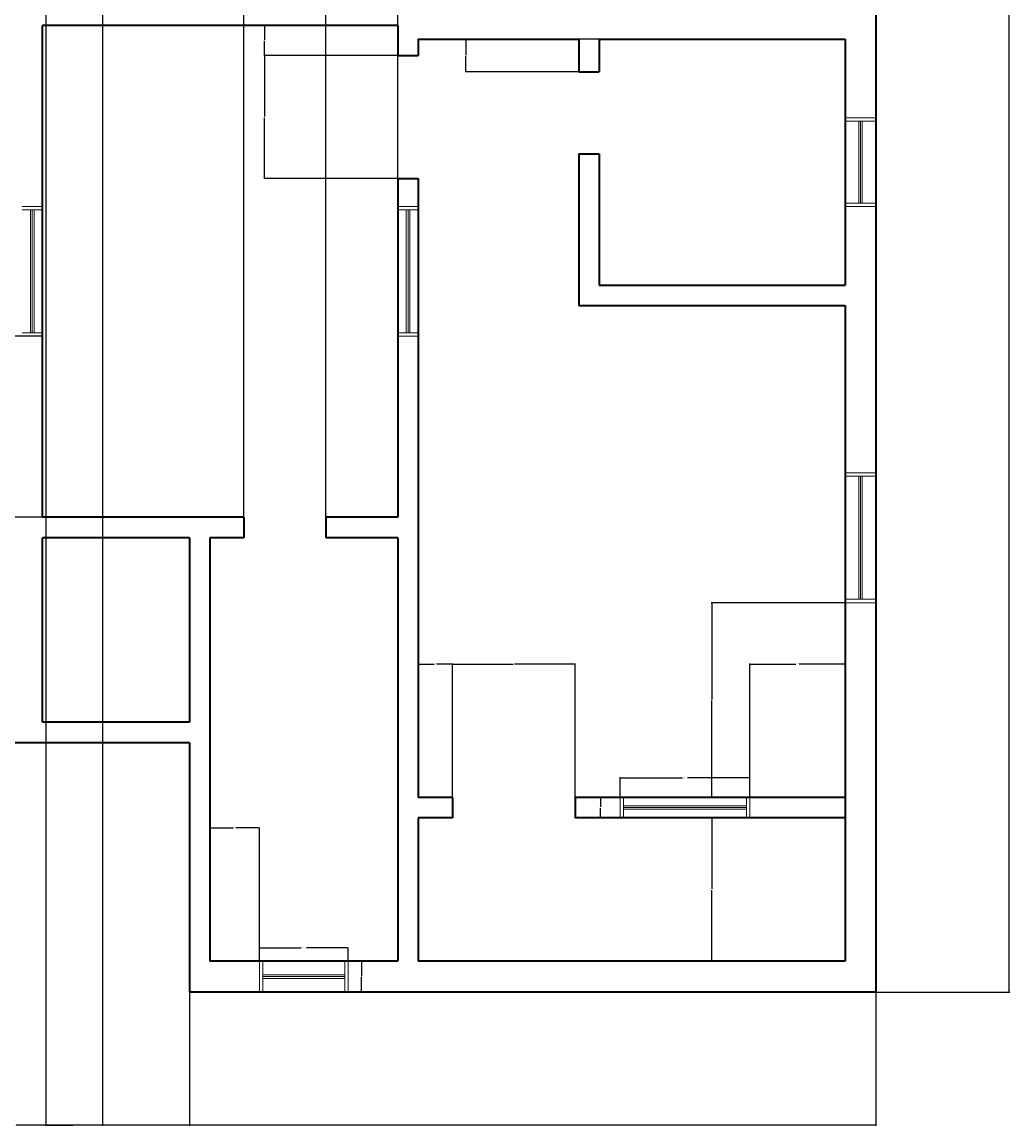
# Model space of a CAD drawing. Units: inches. Extents: x -7288 to -6705, y 7169 to 8028.
# Tile 2 of 5: x -6995 to -6706, y 7169 to 7493. Entities that reach past the tile are written whole.
import ezdxf

# ---------------------------------------------------------------- set-up
doc = ezdxf.new("R2010")
doc.units = ezdxf.units.IN
for name, color, linetype, lineweight in [('A-ANNO-DIMS', 2, 'Continuous', 18), ('A-GLAZ', 2, 'Continuous', 18), ('A-WALL', 1, 'Continuous', 35)]:
    doc.layers.add(name, color=color, linetype=linetype, lineweight=lineweight)
doc.styles.get("Standard").update_dxf_attribs({"font": 'arial.ttf'})
doc.dimstyles.get("Standard").update_dxf_attribs({"dimtxt": 0.18, "dimasz": 0.18, "dimexe": 0.18, "dimexo": 0.0625, "dimgap": 0.09, "dimtad": 0, "dimtih": 1, "dimtoh": 1, "dimdec": 4, "dimzin": 0, "dimdsep": 46, "dimtxsty": 'Standard', "dimcen": 0.09, "dimadec": 0, "dimazin": 0, "dimtfac": 1, "dimtdec": 4, "dimtofl": 0, "dimtmove": 0, "dimatfit": 3, "dimfxl": 1, "dimtolj": 1, "dimtzin": 0, "dimarcsym": 0})

# ---------------------------------------------------------------- blocks, each defined once
blk = doc.blocks.new('WIN-36IN-WALL9')
for p, q in [((0, 38), (9, 38)), ((0, 37), (9, 37)), ((4, 1), (4, 37)), ((4.5, 1), (4.5, 37)), ((5, 1), (5, 37)), ((0, 1), (9, 1)), ((0, 0), (9, 0))]:
    blk.add_line(p, q)
blk = doc.blocks.new('WIN-24IN-WALL9')
for p, q in [((0, 26), (9, 26)), ((0, 25), (9, 25)), ((4, 1), (4, 25)), ((4.5, 1), (4.5, 25)), ((5, 1), (5, 25)), ((0, 1), (9, 1)), ((0, 0), (9, 0))]:
    blk.add_line(p, q)
blk = doc.blocks.new('WIN-36IN-WALL6')
for p, q in [((0, 6), (0, 0)), ((1, 6), (1, 0)), ((1, 3.5), (37, 3.5)), ((37, 6), (37, 0)), ((38, 6), (38, 0)), ((1, 3), (37, 3)), ((1, 2.5), (37, 2.5))]:
    blk.add_line(p, q)
blk = doc.blocks.new('*D89')
at = {"layer": 'A-ANNO-DIMS', "color": 0, "lineweight": -2, "transparency": 16777216}
for p, q in [((-6925.34, 7217.59), (-6925.34, 7221.61)), ((-6925.16, 7221.43), (-6913.1, 7221.43)), ((-6899.52, 7221.43), (-6911.58, 7221.43)), ((-6899.34, 7217.59), (-6899.34, 7221.61))]:
    blk.add_line(p, q, dxfattribs=at)
at = {"layer": 'A-ANNO-DIMS', "color": 0, "transparency": 16777216}
for points in [[(-6925.16, 7221.46), (-6925.16, 7221.4), (-6925.34, 7221.43)], [(-6899.52, 7221.46), (-6899.52, 7221.4), (-6899.34, 7221.43)]]:
    blk.add_solid(points, dxfattribs=at)
at = {"layer": 'Defpoints', "color": 0, "transparency": 16777216}
for p in [(-6899.34, 7221.43), (-6925.34, 7217.53), (-6899.34, 7217.53)]:
    blk.add_point(p, dxfattribs=at)
at = {"layer": 'A-ANNO-DIMS', "color": 0, "transparency": 16777216, "insert": (-6912.34, 7221.43), "char_height": 0.18, "attachment_point": 5}
blk.add_mtext('\\A1;W2 26 TYP.', dxfattribs=at)
blk = doc.blocks.new('*D90')
at = {"layer": 'A-ANNO-DIMS', "color": 0, "lineweight": -2, "transparency": 16777216}
for p, q in [((-6899.28, 7217.53), (-6895.26, 7217.53)), ((-6895.44, 7217.35), (-6895.44, 7213.21)), ((-6895.44, 7208.71), (-6895.44, 7212.85)), ((-6899.28, 7208.53), (-6895.26, 7208.53))]:
    blk.add_line(p, q, dxfattribs=at)
at = {"layer": 'A-ANNO-DIMS', "color": 0, "transparency": 16777216}
for points in [[(-6895.47, 7217.35), (-6895.41, 7217.35), (-6895.44, 7217.53)], [(-6895.47, 7208.71), (-6895.41, 7208.71), (-6895.44, 7208.53)]]:
    blk.add_solid(points, dxfattribs=at)
at = {"layer": 'Defpoints', "color": 0, "transparency": 16777216}
for p in [(-6899.34, 7217.53), (-6899.34, 7208.53), (-6895.44, 7208.53)]:
    blk.add_point(p, dxfattribs=at)
at = {"layer": 'A-ANNO-DIMS', "color": 0, "transparency": 16777216, "insert": (-6895.44, 7213.03), "char_height": 0.18, "attachment_point": 5}
blk.add_mtext('\\A1;9 TYP.', dxfattribs=at)
blk = doc.blocks.new('*D91')
at = {"layer": 'A-ANNO-DIMS', "color": 0, "lineweight": -2, "transparency": 16777216}
for p, q in [((-6819.77, 7265.59), (-6819.77, 7271.41)), ((-6819.59, 7271.23), (-6801.52, 7271.23)), ((-6781.95, 7271.23), (-6800.01, 7271.23)), ((-6781.77, 7265.59), (-6781.77, 7271.41))]:
    blk.add_line(p, q, dxfattribs=at)
at = {"layer": 'A-ANNO-DIMS', "color": 0, "transparency": 16777216}
for points in [[(-6819.59, 7271.26), (-6819.59, 7271.2), (-6819.77, 7271.23)], [(-6781.95, 7271.26), (-6781.95, 7271.2), (-6781.77, 7271.23)]]:
    blk.add_solid(points, dxfattribs=at)
at = {"layer": 'Defpoints', "color": 0, "transparency": 16777216}
for p in [(-6781.77, 7271.23), (-6819.77, 7265.53), (-6781.77, 7265.53)]:
    blk.add_point(p, dxfattribs=at)
at = {"layer": 'A-ANNO-DIMS', "color": 0, "transparency": 16777216, "insert": (-6800.77, 7271.23), "char_height": 0.18, "attachment_point": 5}
blk.add_mtext('\\A1;W3 38 TYP.', dxfattribs=at)
blk = doc.blocks.new('*D92')
at = {"layer": 'A-ANNO-DIMS', "color": 0, "lineweight": -2, "transparency": 16777216}
for p, q in [((-6819.83, 7265.53), (-6825.65, 7265.53)), ((-6825.47, 7265.35), (-6825.47, 7262.71)), ((-6819.83, 7259.53), (-6825.65, 7259.53)), ((-6825.47, 7259.71), (-6825.47, 7262.35))]:
    blk.add_line(p, q, dxfattribs=at)
at = {"layer": 'A-ANNO-DIMS', "color": 0, "transparency": 16777216}
for points in [[(-6825.5, 7265.35), (-6825.44, 7265.35), (-6825.47, 7265.53)], [(-6825.5, 7259.71), (-6825.44, 7259.71), (-6825.47, 7259.53)]]:
    blk.add_solid(points, dxfattribs=at)
at = {"layer": 'Defpoints', "color": 0, "transparency": 16777216}
for p in [(-6825.47, 7265.53), (-6819.77, 7265.53), (-6819.77, 7259.53)]:
    blk.add_point(p, dxfattribs=at)
at = {"layer": 'A-ANNO-DIMS', "color": 0, "transparency": 16777216, "insert": (-6825.47, 7262.53), "char_height": 0.18, "attachment_point": 5}
blk.add_mtext('\\A1;6 TYP.', dxfattribs=at)
blk = doc.blocks.new('*D93')
at = {"layer": 'A-ANNO-DIMS', "color": 0, "lineweight": -2, "transparency": 16777216}
for p, q in [((-7248.84, 7208.47), (-7248.84, 7169.32)), ((-6744.84, 7208.47), (-6744.84, 7169.32)), ((-7248.66, 7169.5), (-6997.13, 7169.5)), ((-6745.02, 7169.5), (-6996.55, 7169.5))]:
    blk.add_line(p, q, dxfattribs=at)
at = {"layer": 'A-ANNO-DIMS', "color": 0, "transparency": 16777216}
for points in [[(-7248.66, 7169.53), (-7248.66, 7169.47), (-7248.84, 7169.5)], [(-6745.02, 7169.53), (-6745.02, 7169.47), (-6744.84, 7169.5)]]:
    blk.add_solid(points, dxfattribs=at)
at = {"layer": 'Defpoints', "color": 0, "transparency": 16777216}
for p in [(-7248.84, 7208.53), (-6744.84, 7208.53), (-6744.84, 7169.5)]:
    blk.add_point(p, dxfattribs=at)
at = {"layer": 'A-ANNO-DIMS', "color": 0, "transparency": 16777216, "insert": (-6996.84, 7169.5), "char_height": 0.18, "attachment_point": 5}
blk.add_mtext('\\A1;504', dxfattribs=at)
blk = doc.blocks.new('*D94')
at = {"layer": 'A-ANNO-DIMS', "color": 0, "lineweight": -2, "transparency": 16777216}
for p, q in [((-6802.78, 7988.53), (-6705.63, 7988.53)), ((-6705.81, 7988.35), (-6705.81, 7598.71)), ((-6705.81, 7208.71), (-6705.81, 7598.35)), ((-6744.78, 7208.53), (-6705.63, 7208.53))]:
    blk.add_line(p, q, dxfattribs=at)
at = {"layer": 'A-ANNO-DIMS', "color": 0, "transparency": 16777216}
for points in [[(-6705.84, 7988.35), (-6705.78, 7988.35), (-6705.81, 7988.53)], [(-6705.84, 7208.71), (-6705.78, 7208.71), (-6705.81, 7208.53)]]:
    blk.add_solid(points, dxfattribs=at)
at = {"layer": 'Defpoints', "color": 0, "transparency": 16777216}
for p in [(-6802.84, 7988.53), (-6705.81, 7988.53), (-6744.84, 7208.53)]:
    blk.add_point(p, dxfattribs=at)
at = {"layer": 'A-ANNO-DIMS', "color": 0, "transparency": 16777216, "insert": (-6705.81, 7598.53), "char_height": 0.18, "attachment_point": 5}
blk.add_mtext('\\A1;780', dxfattribs=at)
blk = doc.blocks.new('*D101')
at = {"layer": 'A-ANNO-DIMS', "color": 0, "lineweight": -2, "transparency": 16777216}
for p, q in [((-7047.84, 7208.47), (-7047.84, 7169.32)), ((-6945.84, 7208.47), (-6945.84, 7169.32)), ((-7047.66, 7169.5), (-6997.12, 7169.5)), ((-6946.02, 7169.5), (-6996.56, 7169.5))]:
    blk.add_line(p, q, dxfattribs=at)
at = {"layer": 'A-ANNO-DIMS', "color": 0, "transparency": 16777216}
for points in [[(-7047.66, 7169.53), (-7047.66, 7169.47), (-7047.84, 7169.5)], [(-6946.02, 7169.53), (-6946.02, 7169.47), (-6945.84, 7169.5)]]:
    blk.add_solid(points, dxfattribs=at)
at = {"layer": 'Defpoints', "color": 0, "transparency": 16777216}
for p in [(-7047.84, 7208.53), (-6945.84, 7208.53), (-6945.84, 7169.5)]:
    blk.add_point(p, dxfattribs=at)
at = {"layer": 'A-ANNO-DIMS', "color": 0, "transparency": 16777216, "insert": (-6996.84, 7169.5), "char_height": 0.18, "attachment_point": 5}
blk.add_mtext('\\A1;102', dxfattribs=at)
blk = doc.blocks.new('*D115')
at = {"layer": 'A-ANNO-DIMS', "color": 0, "lineweight": -2, "transparency": 16777216}
for p, q in [((-6971.26, 7899.49), (-6971.26, 7169.32)), ((-6987.84, 7886.47), (-6987.84, 7169.32)), ((-6987.66, 7169.5), (-6980.01, 7169.5)), ((-6971.44, 7169.5), (-6979.1, 7169.5))]:
    blk.add_line(p, q, dxfattribs=at)
at = {"layer": 'A-ANNO-DIMS', "color": 0, "transparency": 16777216}
for points in [[(-6987.66, 7169.53), (-6987.66, 7169.47), (-6987.84, 7169.5)], [(-6971.44, 7169.53), (-6971.44, 7169.47), (-6971.26, 7169.5)]]:
    blk.add_solid(points, dxfattribs=at)
at = {"layer": 'Defpoints', "color": 0, "transparency": 16777216}
for p in [(-6971.26, 7899.55), (-6987.84, 7886.53), (-6971.26, 7169.5)]:
    blk.add_point(p, dxfattribs=at)
at = {"layer": 'A-ANNO-DIMS', "color": 0, "transparency": 16777216, "insert": (-6979.55, 7169.5), "char_height": 0.18, "attachment_point": 5}
blk.add_mtext('\\A1;16.578', dxfattribs=at)
blk = doc.blocks.new('*D143')
at = {"layer": 'A-ANNO-DIMS', "color": 0, "lineweight": -2, "transparency": 16777216}
for p, q in [((-6753.9, 7259.53), (-6793.05, 7259.53)), ((-6792.87, 7259.35), (-6792.87, 7238.71)), ((-6792.87, 7217.71), (-6792.87, 7238.35)), ((-6753.9, 7217.53), (-6793.05, 7217.53))]:
    blk.add_line(p, q, dxfattribs=at)
at = {"layer": 'A-ANNO-DIMS', "color": 0, "transparency": 16777216}
for points in [[(-6792.9, 7259.35), (-6792.84, 7259.35), (-6792.87, 7259.53)], [(-6792.9, 7217.71), (-6792.84, 7217.71), (-6792.87, 7217.53)]]:
    blk.add_solid(points, dxfattribs=at)
at = {"layer": 'Defpoints', "color": 0, "transparency": 16777216}
for p in [(-6792.87, 7259.53), (-6753.84, 7259.53), (-6753.84, 7217.53)]:
    blk.add_point(p, dxfattribs=at)
at = {"layer": 'A-ANNO-DIMS', "color": 0, "transparency": 16777216, "insert": (-6792.87, 7238.53), "char_height": 0.18, "attachment_point": 5}
blk.add_mtext('\\A1;42', dxfattribs=at)
blk = doc.blocks.new('*D153')
at = {"layer": 'A-ANNO-DIMS', "color": 0, "lineweight": -2, "transparency": 16777216}
for p, q in [((-6753.9, 7322.53), (-6793.05, 7322.53)), ((-6792.87, 7322.35), (-6792.87, 7294.21)), ((-6792.87, 7265.71), (-6792.87, 7293.85)), ((-6753.9, 7265.53), (-6793.05, 7265.53))]:
    blk.add_line(p, q, dxfattribs=at)
at = {"layer": 'A-ANNO-DIMS', "color": 0, "transparency": 16777216}
for points in [[(-6792.9, 7322.35), (-6792.84, 7322.35), (-6792.87, 7322.53)], [(-6792.9, 7265.71), (-6792.84, 7265.71), (-6792.87, 7265.53)]]:
    blk.add_solid(points, dxfattribs=at)
at = {"layer": 'Defpoints', "color": 0, "transparency": 16777216}
for p in [(-6792.87, 7322.53), (-6753.84, 7322.53), (-6753.84, 7265.53)]:
    blk.add_point(p, dxfattribs=at)
at = {"layer": 'A-ANNO-DIMS', "color": 0, "transparency": 16777216, "insert": (-6792.87, 7294.03), "char_height": 0.18, "attachment_point": 5}
blk.add_mtext('\\A1;57', dxfattribs=at)
blk = doc.blocks.new('*D154')
at = {"layer": 'A-ANNO-DIMS', "color": 0, "lineweight": -2, "transparency": 16777216}
for p, q in [((-6905.9, 7347.59), (-6905.9, 8027.74)), ((-6905.72, 8027.56), (-6895.77, 8027.56)), ((-6885.02, 8027.56), (-6894.97, 8027.56)), ((-6884.84, 7347.59), (-6884.84, 8027.74))]:
    blk.add_line(p, q, dxfattribs=at)
at = {"layer": 'A-ANNO-DIMS', "color": 0, "transparency": 16777216}
for points in [[(-6905.72, 8027.59), (-6905.72, 8027.53), (-6905.9, 8027.56)], [(-6885.02, 8027.59), (-6885.02, 8027.53), (-6884.84, 8027.56)]]:
    blk.add_solid(points, dxfattribs=at)
at = {"layer": 'Defpoints', "color": 0, "transparency": 16777216}
for p in [(-6884.84, 8027.56), (-6905.9, 7347.53), (-6884.84, 7347.53)]:
    blk.add_point(p, dxfattribs=at)
at = {"layer": 'A-ANNO-DIMS', "color": 0, "transparency": 16777216, "insert": (-6895.37, 8027.56), "char_height": 0.18, "attachment_point": 5}
blk.add_mtext('\\A1;21.06', dxfattribs=at)
blk = doc.blocks.new('*D155')
at = {"layer": 'A-ANNO-DIMS', "color": 0, "lineweight": -2, "transparency": 16777216}
for p, q in [((-6929.9, 7347.59), (-6929.9, 8027.74)), ((-6929.72, 8027.56), (-6918.12, 8027.56)), ((-6906.08, 8027.56), (-6917.68, 8027.56)), ((-6905.9, 7347.59), (-6905.9, 8027.74))]:
    blk.add_line(p, q, dxfattribs=at)
at = {"layer": 'A-ANNO-DIMS', "color": 0, "transparency": 16777216}
for points in [[(-6929.72, 8027.59), (-6929.72, 8027.53), (-6929.9, 8027.56)], [(-6906.08, 8027.59), (-6906.08, 8027.53), (-6905.9, 8027.56)]]:
    blk.add_solid(points, dxfattribs=at)
at = {"layer": 'Defpoints', "color": 0, "transparency": 16777216}
for p in [(-6905.9, 8027.56), (-6929.9, 7347.53), (-6905.9, 7347.53)]:
    blk.add_point(p, dxfattribs=at)
at = {"layer": 'A-ANNO-DIMS', "color": 0, "transparency": 16777216, "insert": (-6917.9, 8027.56), "char_height": 0.18, "attachment_point": 5}
blk.add_mtext('\\A1;24', dxfattribs=at)
blk = doc.blocks.new('*D159')
at = {"layer": 'A-ANNO-DIMS', "color": 0, "lineweight": -2, "transparency": 16777216}
for p, q in [((-6939.84, 7217.59), (-6939.84, 7256.74)), ((-6939.66, 7256.56), (-6932.91, 7256.56)), ((-6925.52, 7256.56), (-6932.27, 7256.56)), ((-6925.34, 7217.59), (-6925.34, 7256.74))]:
    blk.add_line(p, q, dxfattribs=at)
at = {"layer": 'A-ANNO-DIMS', "color": 0, "transparency": 16777216}
for points in [[(-6939.66, 7256.59), (-6939.66, 7256.53), (-6939.84, 7256.56)], [(-6925.52, 7256.59), (-6925.52, 7256.53), (-6925.34, 7256.56)]]:
    blk.add_solid(points, dxfattribs=at)
at = {"layer": 'Defpoints', "color": 0, "transparency": 16777216}
for p in [(-6925.34, 7256.56), (-6939.84, 7217.53), (-6925.34, 7217.53)]:
    blk.add_point(p, dxfattribs=at)
at = {"layer": 'A-ANNO-DIMS', "color": 0, "transparency": 16777216, "insert": (-6932.59, 7256.56), "char_height": 0.18, "attachment_point": 5}
blk.add_mtext('\\A1;14.5', dxfattribs=at)
blk = doc.blocks.new('*D160')
at = {"layer": 'A-ANNO-DIMS', "color": 0, "lineweight": -2, "transparency": 16777216}
for p, q in [((-6988.9, 7400.53), (-7028.05, 7400.53)), ((-7027.87, 7400.35), (-7027.87, 7374.21)), ((-7027.87, 7347.71), (-7027.87, 7373.85)), ((-6988.9, 7347.53), (-7028.05, 7347.53))]:
    blk.add_line(p, q, dxfattribs=at)
at = {"layer": 'A-ANNO-DIMS', "color": 0, "transparency": 16777216}
for points in [[(-7027.9, 7400.35), (-7027.84, 7400.35), (-7027.87, 7400.53)], [(-7027.9, 7347.71), (-7027.84, 7347.71), (-7027.87, 7347.53)]]:
    blk.add_solid(points, dxfattribs=at)
at = {"layer": 'Defpoints', "color": 0, "transparency": 16777216}
for p in [(-7027.87, 7400.53), (-6988.84, 7400.53), (-6988.84, 7347.53)]:
    blk.add_point(p, dxfattribs=at)
at = {"layer": 'A-ANNO-DIMS', "color": 0, "transparency": 16777216, "insert": (-7027.87, 7374.03), "char_height": 0.18, "attachment_point": 5}
blk.add_mtext('\\A1;53', dxfattribs=at)
blk = doc.blocks.new('*D162')
at = {"layer": 'A-ANNO-DIMS', "color": 0, "lineweight": -2, "transparency": 16777216}
for p, q in [((-6781.77, 7265.59), (-6781.77, 7304.74)), ((-6781.59, 7304.56), (-6768.27, 7304.56)), ((-6754.02, 7304.56), (-6767.34, 7304.56)), ((-6753.84, 7265.59), (-6753.84, 7304.74))]:
    blk.add_line(p, q, dxfattribs=at)
at = {"layer": 'A-ANNO-DIMS', "color": 0, "transparency": 16777216}
for points in [[(-6781.59, 7304.59), (-6781.59, 7304.53), (-6781.77, 7304.56)], [(-6754.02, 7304.59), (-6754.02, 7304.53), (-6753.84, 7304.56)]]:
    blk.add_solid(points, dxfattribs=at)
at = {"layer": 'Defpoints', "color": 0, "transparency": 16777216}
for p in [(-6753.84, 7304.56), (-6781.77, 7265.53), (-6753.84, 7265.53)]:
    blk.add_point(p, dxfattribs=at)
at = {"layer": 'A-ANNO-DIMS', "color": 0, "transparency": 16777216, "insert": (-6767.8, 7304.56), "char_height": 0.18, "attachment_point": 5}
blk.add_mtext('\\A1;27.925', dxfattribs=at)
blk = doc.blocks.new('*D167')
at = {"layer": 'A-ANNO-DIMS', "color": 0, "lineweight": -2, "transparency": 16777216}
for p, q in [((-6884.9, 7482.7), (-6924.05, 7482.7)), ((-6923.87, 7482.52), (-6923.87, 7464.88)), ((-6923.87, 7446.88), (-6923.87, 7464.52)), ((-6884.9, 7446.7), (-6924.05, 7446.7))]:
    blk.add_line(p, q, dxfattribs=at)
at = {"layer": 'A-ANNO-DIMS', "color": 0, "transparency": 16777216}
for points in [[(-6923.9, 7482.52), (-6923.84, 7482.52), (-6923.87, 7482.7)], [(-6923.9, 7446.88), (-6923.84, 7446.88), (-6923.87, 7446.7)]]:
    blk.add_solid(points, dxfattribs=at)
at = {"layer": 'Defpoints', "color": 0, "transparency": 16777216}
for p in [(-6923.87, 7482.7), (-6884.84, 7482.7), (-6884.84, 7446.7)]:
    blk.add_point(p, dxfattribs=at)
at = {"layer": 'A-ANNO-DIMS', "color": 0, "transparency": 16777216, "insert": (-6923.87, 7464.7), "char_height": 0.18, "attachment_point": 5}
blk.add_mtext('\\A1;36', dxfattribs=at)
blk = doc.blocks.new('*D168')
at = {"layer": 'A-ANNO-DIMS', "color": 0, "lineweight": -2, "transparency": 16777216}
for p, q in [((-6884.9, 7491.53), (-6924.05, 7491.53)), ((-6923.87, 7491.35), (-6923.87, 7487.3)), ((-6923.87, 7482.88), (-6923.87, 7486.93)), ((-6884.9, 7482.7), (-6924.05, 7482.7))]:
    blk.add_line(p, q, dxfattribs=at)
at = {"layer": 'A-ANNO-DIMS', "color": 0, "transparency": 16777216}
for points in [[(-6923.9, 7491.35), (-6923.84, 7491.35), (-6923.87, 7491.53)], [(-6923.9, 7482.88), (-6923.84, 7482.88), (-6923.87, 7482.7)]]:
    blk.add_solid(points, dxfattribs=at)
at = {"layer": 'Defpoints', "color": 0, "transparency": 16777216}
for p in [(-6923.87, 7491.53), (-6884.84, 7491.53), (-6884.84, 7482.7)]:
    blk.add_point(p, dxfattribs=at)
at = {"layer": 'A-ANNO-DIMS', "color": 0, "transparency": 16777216, "insert": (-6923.87, 7487.11), "char_height": 0.18, "attachment_point": 5}
blk.add_mtext('\\A1;8.834', dxfattribs=at)
blk = doc.blocks.new('*D171')
at = {"layer": 'A-ANNO-DIMS', "color": 0, "lineweight": -2, "transparency": 16777216}
for p, q in [((-6825.9, 7487.53), (-6865.05, 7487.53)), ((-6864.87, 7487.35), (-6864.87, 7482.94)), ((-6864.87, 7478.17), (-6864.87, 7482.58)), ((-6825.9, 7477.99), (-6865.05, 7477.99))]:
    blk.add_line(p, q, dxfattribs=at)
at = {"layer": 'A-ANNO-DIMS', "color": 0, "transparency": 16777216}
for points in [[(-6864.9, 7487.35), (-6864.84, 7487.35), (-6864.87, 7487.53)], [(-6864.9, 7478.17), (-6864.84, 7478.17), (-6864.87, 7477.99)]]:
    blk.add_solid(points, dxfattribs=at)
at = {"layer": 'Defpoints', "color": 0, "transparency": 16777216}
for p in [(-6864.87, 7487.53), (-6825.84, 7487.53), (-6825.84, 7477.99)]:
    blk.add_point(p, dxfattribs=at)
at = {"layer": 'A-ANNO-DIMS', "color": 0, "transparency": 16777216, "insert": (-6864.87, 7482.76), "char_height": 0.18, "attachment_point": 5}
blk.add_mtext('\\A1;9.545', dxfattribs=at)
blk = doc.blocks.new('*D174')
at = {"layer": 'A-ANNO-DIMS', "color": 0, "lineweight": -2, "transparency": 16777216}
for p, q in [((-6878.84, 7265.59), (-6878.84, 7304.74)), ((-6878.66, 7304.56), (-6874.17, 7304.56)), ((-6869.04, 7304.56), (-6873.53, 7304.56)), ((-6868.86, 7265.59), (-6868.86, 7304.74))]:
    blk.add_line(p, q, dxfattribs=at)
at = {"layer": 'A-ANNO-DIMS', "color": 0, "transparency": 16777216}
for points in [[(-6878.66, 7304.59), (-6878.66, 7304.53), (-6878.84, 7304.56)], [(-6869.04, 7304.59), (-6869.04, 7304.53), (-6868.86, 7304.56)]]:
    blk.add_solid(points, dxfattribs=at)
at = {"layer": 'Defpoints', "color": 0, "transparency": 16777216}
for p in [(-6868.86, 7304.56), (-6878.84, 7265.53), (-6868.86, 7265.53)]:
    blk.add_point(p, dxfattribs=at)
at = {"layer": 'A-ANNO-DIMS', "color": 0, "transparency": 16777216, "insert": (-6873.85, 7304.56), "char_height": 0.18, "attachment_point": 5}
blk.add_mtext('\\A1;9.98', dxfattribs=at)
blk = doc.blocks.new('*D175')
at = {"layer": 'A-ANNO-DIMS', "color": 0, "lineweight": -2, "transparency": 16777216}
for p, q in [((-6868.86, 7265.59), (-6868.86, 7304.74)), ((-6868.68, 7304.56), (-6851.08, 7304.56)), ((-6833.04, 7304.56), (-6850.64, 7304.56)), ((-6832.86, 7265.59), (-6832.86, 7304.74))]:
    blk.add_line(p, q, dxfattribs=at)
at = {"layer": 'A-ANNO-DIMS', "color": 0, "transparency": 16777216}
for points in [[(-6868.68, 7304.59), (-6868.68, 7304.53), (-6868.86, 7304.56)], [(-6833.04, 7304.59), (-6833.04, 7304.53), (-6832.86, 7304.56)]]:
    blk.add_solid(points, dxfattribs=at)
at = {"layer": 'Defpoints', "color": 0, "transparency": 16777216}
for p in [(-6832.86, 7304.56), (-6868.86, 7265.53), (-6832.86, 7265.53)]:
    blk.add_point(p, dxfattribs=at)
at = {"layer": 'A-ANNO-DIMS', "color": 0, "transparency": 16777216, "insert": (-6850.86, 7304.56), "char_height": 0.18, "attachment_point": 5}
blk.add_mtext('\\A1;36', dxfattribs=at)

msp = doc.modelspace()

# ---------------------------------------------------------------- linework, layer by layer
at = {"layer": 'A-WALL'}
for p, q in [((-6744.8398, 7958.5311), (-6744.8398, 7208.5311)), ((-6884.8398, 7491.5311), (-6988.8398, 7491.5311)), ((-6988.8398, 7347.5311), (-6988.8398, 7491.5311)), ((-6884.8398, 7491.5311), (-6884.8398, 7482.6972)), ((-6878.8398, 7487.5311), (-6831.8398, 7487.5311)), ((-6878.8398, 7487.5311), (-6878.8398, 7482.6972)), ((-6831.8398, 7487.5311), (-6831.8398, 7477.9856)), ((-6825.8398, 7487.5311), (-6825.8398, 7477.9856)), ((-6825.8398, 7487.5311), (-6753.8398, 7487.5311)), ((-6753.8398, 7487.5311), (-6753.8398, 7415.5311)), ((-6884.8398, 7482.6972), (-6878.8398, 7482.6972)), ((-6831.8398, 7477.9856), (-6825.8398, 7477.9856)), ((-6831.8398, 7453.9856), (-6825.8398, 7453.9856)), ((-6831.8398, 7453.9856), (-6831.8398, 7409.5311)), ((-6825.8398, 7453.9856), (-6825.8398, 7415.5311)), ((-6884.8398, 7446.6972), (-6878.8398, 7446.6972)), ((-6884.8398, 7446.6972), (-6884.8398, 7347.5311)), ((-6878.8398, 7446.6972), (-6878.8398, 7341.5311)), ((-6825.8398, 7415.5311), (-6753.8398, 7415.5311)), ((-6831.8398, 7409.5311), (-6753.8398, 7409.5311)), ((-6753.8398, 7409.5311), (-6753.8398, 7341.5311)), ((-6929.9003, 7347.5311), (-6988.8398, 7347.5311)), ((-6929.9003, 7347.5311), (-6929.9003, 7341.5311)), ((-6884.8398, 7347.5311), (-6905.9003, 7347.5311)), ((-6905.9003, 7347.5311), (-6905.9003, 7341.5311)), ((-6988.8398, 7287.5311), (-6988.8398, 7341.5311)), ((-6945.8398, 7341.5311), (-6988.8398, 7341.5311)), ((-6945.8398, 7341.5311), (-6945.8398, 7287.5311)), ((-6939.8398, 7341.5311), (-6939.8398, 7217.5311)), ((-6929.9003, 7341.5311), (-6939.8398, 7341.5311)), ((-6884.8398, 7341.5311), (-6905.9003, 7341.5311)), ((-6884.8398, 7341.5311), (-6884.8398, 7217.5311)), ((-6878.8398, 7341.5311), (-6878.8398, 7265.5311)), ((-6753.8398, 7341.5311), (-6753.8398, 7259.5311)), ((-6945.8398, 7287.5311), (-6988.8398, 7287.5311)), ((-6945.8398, 7281.5311), (-7047.8398, 7281.5311)), ((-6945.8398, 7281.5311), (-6945.8398, 7208.5311)), ((-6868.86, 7265.5311), (-6878.8398, 7265.5311)), ((-6868.86, 7265.5311), (-6868.86, 7259.5311)), ((-6753.8398, 7265.5311), (-6832.86, 7265.5311)), ((-6832.86, 7265.5311), (-6832.86, 7259.5311)), ((-6878.8398, 7259.5311), (-6878.8398, 7217.5311)), ((-6868.86, 7259.5311), (-6878.8398, 7259.5311)), ((-6753.8398, 7259.5311), (-6832.86, 7259.5311)), ((-6753.8398, 7259.5311), (-6753.8398, 7217.5311)), ((-6884.8398, 7217.5311), (-6939.8398, 7217.5311)), ((-6753.8398, 7217.5311), (-6878.8398, 7217.5311)), ((-6744.8398, 7208.5311), (-6945.8398, 7208.5311))]:
    msp.add_line(p, q, dxfattribs=at)

# ---------------------------------------------------------------- block references
at = {"layer": 'A-GLAZ'}
for name, p in [('WIN-24IN-WALL9', (-6753.8398, 7438.5311)), ('WIN-36IN-WALL6', (-6819.7653, 7259.5311))]:
    msp.add_blockref(name, p, dxfattribs=at)
for name, p, rotation in [('WIN-36IN-WALL6', (-6988.8398, 7400.5311), 90.00000000000634), ('WIN-36IN-WALL6', (-6878.8398, 7400.5311), 90.00000000000944), ('WIN-36IN-WALL9', (-6744.8398, 7360.5311), 180), ('WIN-24IN-WALL9', (-6925.3398, 7217.5311), 269.9999999999977)]:
    msp.add_blockref(name, p, dxfattribs=dict(at, rotation=rotation))

# ---------------------------------------------------------------- dimensions: what is measured, and where the dimension line sits
at = {"layer": 'A-ANNO-DIMS'}
for base, p1, p2, override, picture, middle in [((-6905.9003, 8027.5611), (-6929.9003, 7347.5311), (-6905.9003, 7347.5311), {"dimdec": 0, "dimlfac": 1, "dimrnd": 0, "dimzin": 0, "dimdsep": 46, "dimlunit": 2}, '*D155', (-6917.9003, 8027.5611)), ((-6884.8398, 8027.5611), (-6905.9003, 7347.5311), (-6884.8398, 7347.5311), {"dimdec": 2, "dimlfac": 1, "dimrnd": 0, "dimzin": 0, "dimdsep": 46, "dimlunit": 2}, '*D154', (-6895.3701, 8027.5611)), ((-6971.2622, 7169.5011), (-6987.8398, 7886.5311), (-6971.2622, 7899.5515), {"dimdec": 3, "dimlfac": 1, "dimrnd": 0, "dimzin": 0, "dimdsep": 46, "dimlunit": 2}, '*D115', (-6979.551, 7169.5011)), ((-6868.86, 7304.5611), (-6878.8398, 7265.5311), (-6868.86, 7265.5311), {"dimdec": 2, "dimlfac": 1, "dimrnd": 0, "dimzin": 0, "dimdsep": 46, "dimlunit": 2}, '*D174', (-6873.8499, 7304.5611)), ((-6832.86, 7304.5611), (-6868.86, 7265.5311), (-6832.86, 7265.5311), {"dimdec": 0, "dimlfac": 1, "dimrnd": 0, "dimzin": 0, "dimdsep": 46, "dimlunit": 2}, '*D175', (-6850.86, 7304.5611)), ((-6744.8398, 7169.5011), (-7248.8398, 7208.5311), (-6744.8398, 7208.5311), {"dimdec": 0, "dimlfac": 1, "dimrnd": 0, "dimzin": 0, "dimdsep": 46, "dimlunit": 2}, '*D93', (-6996.8398, 7169.5011)), ((-6945.8398, 7169.5011), (-7047.8398, 7208.5311), (-6945.8398, 7208.5311), {"dimdec": 0, "dimlfac": 1, "dimrnd": 0, "dimzin": 0, "dimdsep": 46, "dimlunit": 2}, '*D101', (-6996.8398, 7169.5011))]:
    dim = msp.add_linear_dim(base=base, p1=p1, p2=p2, dimstyle='Standard', override=override, dxfattribs=at)
    dim.commit()
    dim.dimension.update_dxf_attribs({"geometry": picture, "text_midpoint": middle})
for base, p1, p2, angle, override, picture, middle in [((-6705.8098, 7988.5311), (-6744.8398, 7208.5311), (-6802.8398, 7988.5311), 90, {"dimdec": 0, "dimlfac": 1, "dimrnd": 0, "dimzin": 0, "dimdsep": 46, "dimlunit": 2}, '*D94', (-6705.8098, 7598.5311)), ((-6923.8698, 7491.5311), (-6884.8398, 7482.6972), (-6884.8398, 7491.5311), 90, {"dimdec": 3, "dimlfac": 1, "dimrnd": 0, "dimzin": 0, "dimdsep": 46, "dimlunit": 2}, '*D168', (-6923.8698, 7487.1141)), ((-6864.86982, 7487.5311), (-6825.83982, 7477.98563), (-6825.83982, 7487.5311), 90, {"dimdec": 3, "dimlfac": 1, "dimrnd": 0, "dimzin": 0, "dimdsep": 46, "dimlunit": 2}, '*D171', (-6864.86982, 7482.75836)), ((-6923.8698, 7482.6972), (-6884.8398, 7446.6972), (-6884.8398, 7482.6972), 90, {"dimdec": 0, "dimlfac": 1, "dimrnd": 0, "dimzin": 0, "dimdsep": 46, "dimlunit": 2}, '*D167', (-6923.8698, 7464.6972)), ((-7027.8698, 7400.5311), (-6988.8398, 7347.5311), (-6988.8398, 7400.5311), 90, {"dimdec": 0, "dimlfac": 1, "dimrnd": 0, "dimzin": 0, "dimdsep": 46, "dimlunit": 2}, '*D160', (-7027.8698, 7374.0311)), ((-6792.8698, 7322.5311), (-6753.8398, 7265.5311), (-6753.8398, 7322.5311), 90, {"dimdec": 0, "dimlfac": 1, "dimrnd": 0, "dimzin": 0, "dimdsep": 46, "dimlunit": 2}, '*D153', (-6792.8698, 7294.0311)), ((-6753.83982, 7304.5611), (-6781.76526, 7265.5311), (-6753.83982, 7265.5311), 0, {"dimdec": 3, "dimlfac": 1, "dimrnd": 0, "dimzin": 0, "dimdsep": 46, "dimlunit": 2}, '*D162', (-6767.80254, 7304.5611)), ((-6792.8698, 7259.5311), (-6753.8398, 7217.5311), (-6753.8398, 7259.5311), 90, {"dimdec": 0, "dimlfac": 1, "dimrnd": 0, "dimzin": 0, "dimdsep": 46, "dimlunit": 2}, '*D143', (-6792.8698, 7238.5311)), ((-6925.3398, 7256.5611), (-6939.8398, 7217.5311), (-6925.3398, 7217.5311), 0, {"dimdec": 1, "dimlfac": 1, "dimrnd": 0, "dimzin": 0, "dimdsep": 46, "dimlunit": 2}, '*D159', (-6932.5898, 7256.5611))]:
    dim = msp.add_linear_dim(base=base, p1=p1, p2=p2, angle=angle, dimstyle='Standard', override=override, dxfattribs=at)
    dim.commit()
    dim.dimension.update_dxf_attribs({"geometry": picture, "text_midpoint": middle})
for base, p1, p2, text, picture, middle in [((-6781.7653, 7271.2311), (-6819.7653, 7265.5311), (-6781.7653, 7265.5311), 'W3 <> TYP.', '*D91', (-6800.7653, 7271.2311)), ((-6899.3398, 7221.4311), (-6925.3398, 7217.5311), (-6899.3398, 7217.5311), 'W2 <> TYP.', '*D89', (-6912.3398, 7221.4311))]:
    dim = msp.add_linear_dim(base=base, p1=p1, p2=p2, text=text, dimstyle='Standard', override={"dimdec": 0, "dimlfac": 1, "dimrnd": 0, "dimzin": 0, "dimdsep": 46, "dimlunit": 2}, dxfattribs=at)
    dim.commit()
    dim.dimension.update_dxf_attribs({"geometry": picture, "text_midpoint": middle})
for base, p1, p2, angle, picture, middle in [((-6825.4653, 7265.5311), (-6819.7653, 7259.5311), (-6819.7653, 7265.5311), 90, '*D92', (-6825.4653, 7262.5311)), ((-6895.4398, 7208.5311), (-6899.3398, 7217.5311), (-6899.3398, 7208.5311), 270, '*D90', (-6895.4398, 7213.0311))]:
    dim = msp.add_linear_dim(base=base, p1=p1, p2=p2, angle=angle, text='<> TYP.', dimstyle='Standard', override={"dimdec": 0, "dimlfac": 1, "dimrnd": 0, "dimzin": 0, "dimdsep": 46, "dimlunit": 2}, dxfattribs=at)
    dim.commit()
    dim.dimension.update_dxf_attribs({"geometry": picture, "text_midpoint": middle})

doc.saveas('drawing.dxf')
